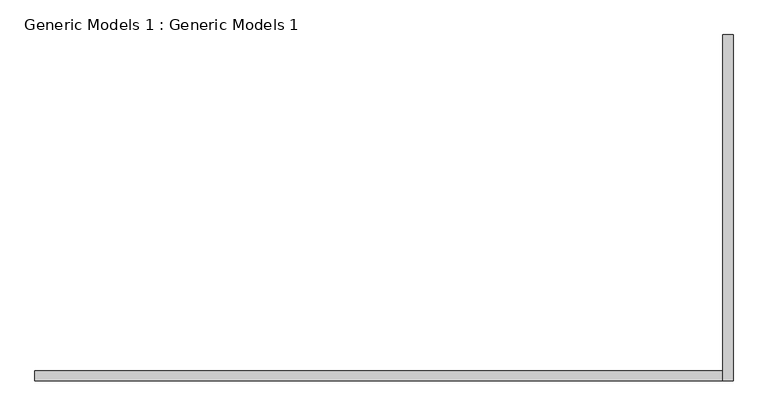
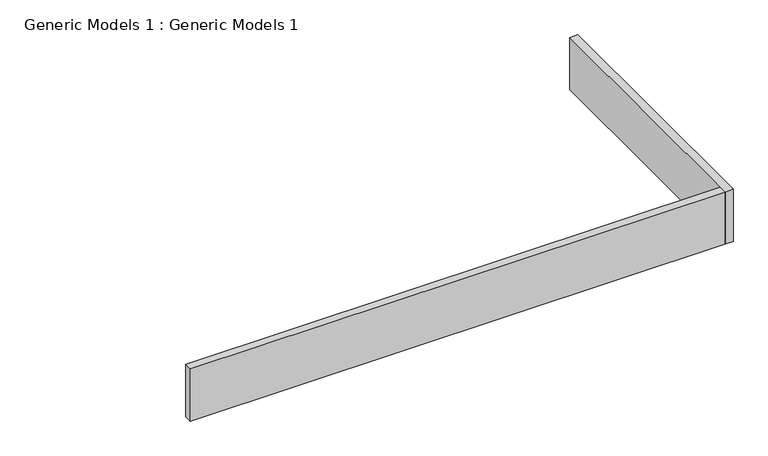
"""IFC4 building model written with IfcOpenShell, lengths in millimetres: proxy geometry, Generic Models 1 : Generic Models 1."""

from ifc_helpers import new_model, si_unit, frame, origin, place, context, project, spatial, polyline, outline, extrude, source, transform, mapped, element, save


def generic_models_1_generic_models_1_a93b3e87(model_context):
    return source(origin(), model_context, "Body", "SweptSolid", [
        extrude(outline(polyline([(-10495.6371373, -2516.661407), (-10495.6371373, -3380.261407), (-10521.0371373, -3380.261407), (-10521.0371373, -2516.661407), (-10495.6371373, -2516.661407)])), frame((0.0, 0.0, 1346.2), z_axis=(0.0, 0.0, 1.0), x_axis=(1.0, 0.0, 0.0)), (0.0, 0.0, 1.0), 177.8),
        extrude(outline(polyline([(-10521.0371373, -3380.261407), (-12235.5371373, -3380.261407), (-12235.5371373, -3354.861407), (-10521.0371373, -3354.861407), (-10521.0371373, -3380.261407)])), frame((0.0, 0.0, 1346.2), z_axis=(0.0, 0.0, 1.0), x_axis=(1.0, 0.0, 0.0)), (0.0, 0.0, 1.0), 177.8),
    ])


if __name__ == "__main__":
    model = new_model("IFC4")
    model_context = context("Model", 3, world=origin())
    ifc_project = project(units=[si_unit("LENGTHUNIT", "METRE", prefix="MILLI")], contexts=[model_context])
    site = spatial("IfcSite", under=ifc_project)
    building = spatial("IfcBuilding", under=site)
    placement = place(None, origin())
    generic_models_1_generic_models_1_shape = generic_models_1_generic_models_1_a93b3e87(model_context)
    element("IfcBuildingElementProxy", 1, Name="Generic Models 1 : Generic Models 1", ObjectType="Generic Models 1 : Generic Models 1", at=placement, inside=building, context=model_context, shape_type="MappedRepresentation", body=[
        mapped(generic_models_1_generic_models_1_shape, transform((0.0, 0.0, 0.0), x_axis=(1.0, 0.0, 0.0), y_axis=(0.0, 1.0, 0.0), z_axis=(0.0, 0.0, 1.0))),
    ])
    save(model, "model.ifc")

# Revit data of these elements
# Element 1 (IfcBuildingElementProxy, "Generic Models 1 : Generic Models 1")
#   Materials on its faces: "Gypsum Wall Board"
# Materials
#   "Gypsum Wall Board": class "Generic", colour RGB 127 127 127, transparency 0, Description = "Gypsum Wall Board", Cost = 0
